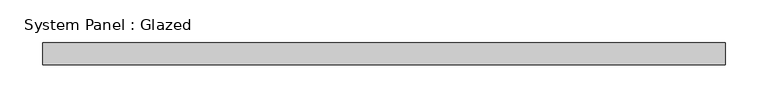
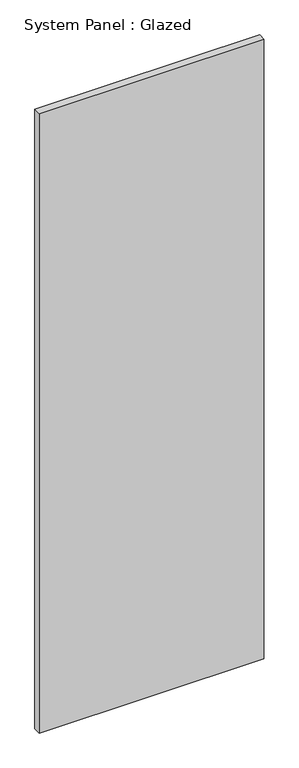
"""IFC4 building model written with IfcOpenShell, lengths in millimetres: plate geometry, System Panel : Glazed."""

from ifc_helpers import new_model, si_unit, origin, origin_with_axes, place, context, project, spatial, polyline, outline, extrude, source, transform, mapped, element, save


def system_panel_glazed_55ca81fc(model_context):
    return source(origin(), model_context, "Body", "SweptSolid", [
        extrude(outline(polyline([(397.9333333, 19.05), (-397.9333333, 19.05), (-397.9333333, 44.45), (397.9333333, 44.45), (397.9333333, 19.05)])), origin_with_axes(), (0.0, 0.0, 1.0), 2317.75),
    ])


if __name__ == "__main__":
    model = new_model("IFC4")
    model_context = context("Model", 3, world=origin())
    ifc_project = project(units=[si_unit("LENGTHUNIT", "METRE", prefix="MILLI")], contexts=[model_context])
    site = spatial("IfcSite", under=ifc_project)
    building = spatial("IfcBuilding", under=site)
    placement = place(None, origin())
    system_panel_glazed_shape = system_panel_glazed_55ca81fc(model_context)
    element("IfcPlate", 1, ObjectType="System Panel : Glazed", at=placement, inside=building, context=model_context, shape_type="MappedRepresentation", body=[
        mapped(system_panel_glazed_shape, transform((0.0, 0.0, 0.0), x_axis=(1.0, 0.0, 0.0), y_axis=(0.0, 1.0, 0.0), z_axis=(0.0, 0.0, 1.0))),
    ])
    save(model, "model.ifc")

# Revit data of these elements
# Type "System Panel : Glazed"
#   Construction Type Id = "GSP4R"
#   Analytic Construction = "1/8 in Pilkington single glazing"
#   Visual Light Transmittance = 0.9
#   Solar Heat Gain Coefficient = 0.86
#   Heat Transfer Coefficient (U) = 1.18115 BTU/(h·ft²·°F)
# Element 1 (IfcPlate, "System Panel : Glazed")
#   Materials on its faces: "Glass"
# Materials
#   "Glass": class "Glass", colour RGB 0 128 192, transparency 0.75, Description = "Soda Lime Glass", Cost = 0
